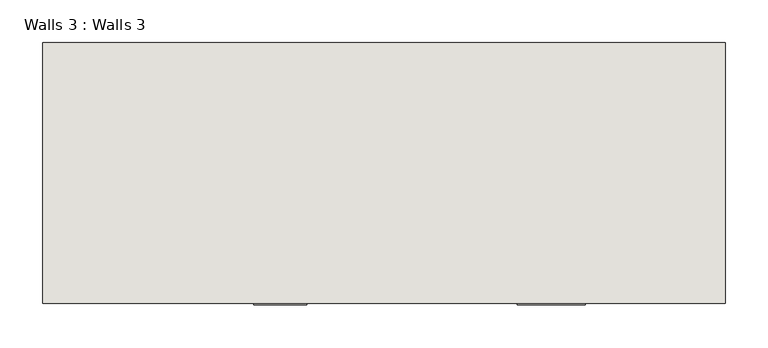
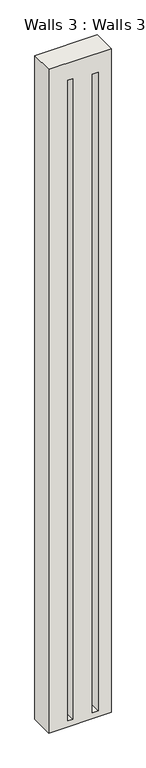
"""IFC4 building model written with IfcOpenShell, lengths in millimetres: wall geometry, Walls 3 : Walls 3."""

from ifc_helpers import new_model, si_unit, frame, origin, place, context, project, spatial, polyline, outline, extrude, source, transform, mapped, element, save


def walls_3_walls_3_54e0ac51(model_context):
    return source(origin(), model_context, "Body", "SweptSolid", [
        extrude(outline(polyline([(8970.5998721, -5378.364671), (8970.5998721, -6175.1407032), (0.0, -6175.1407032), (0.0, -5378.364671), (8970.5998721, -5378.364671)]), holes=[polyline([(8734.4888267, -5867.1704194), (77.6994037, -5867.1704194), (77.6994037, -5928.6990432), (8734.4888267, -5928.6990432), (8734.4888267, -5867.1704194)]), polyline([(8706.4756518, -5541.5145177), (77.6994037, -5541.5145177), (77.6994037, -5621.2293332), (8706.4756518, -5621.2293332), (8706.4756518, -5541.5145177)])]), frame((0.0, 3251.3956099, 0.0), z_axis=(0.0, 1.0, 0.0), x_axis=(0.0, 0.0, 1.0)), (0.0, 0.0, 1.0), 304.8),
    ])


if __name__ == "__main__":
    model = new_model("IFC4")
    model_context = context("Model", 3, world=origin())
    ifc_project = project(units=[si_unit("LENGTHUNIT", "METRE", prefix="MILLI")], contexts=[model_context])
    site = spatial("IfcSite", under=ifc_project)
    building = spatial("IfcBuilding", under=site)
    placement = place(None, origin())
    walls_3_walls_3_shape = walls_3_walls_3_54e0ac51(model_context)
    element("IfcWall", 1, ObjectType="Walls 3 : Walls 3", at=placement, inside=building, context=model_context, shape_type="MappedRepresentation", body=[
        mapped(walls_3_walls_3_shape, transform((0.0, 0.0, 0.0), x_axis=(1.0, 0.0, 0.0), y_axis=(0.0, 1.0, 0.0), z_axis=(0.0, 0.0, 1.0))),
    ])
    save(model, "model.ifc")

# Revit data of these elements
# Element 1 (IfcWall, "Walls 3 : Walls 3")
#   Materials on its faces: "Default Wall"
# Materials
#   "Default Wall": colour RGB 80 80 80, transparency 0
